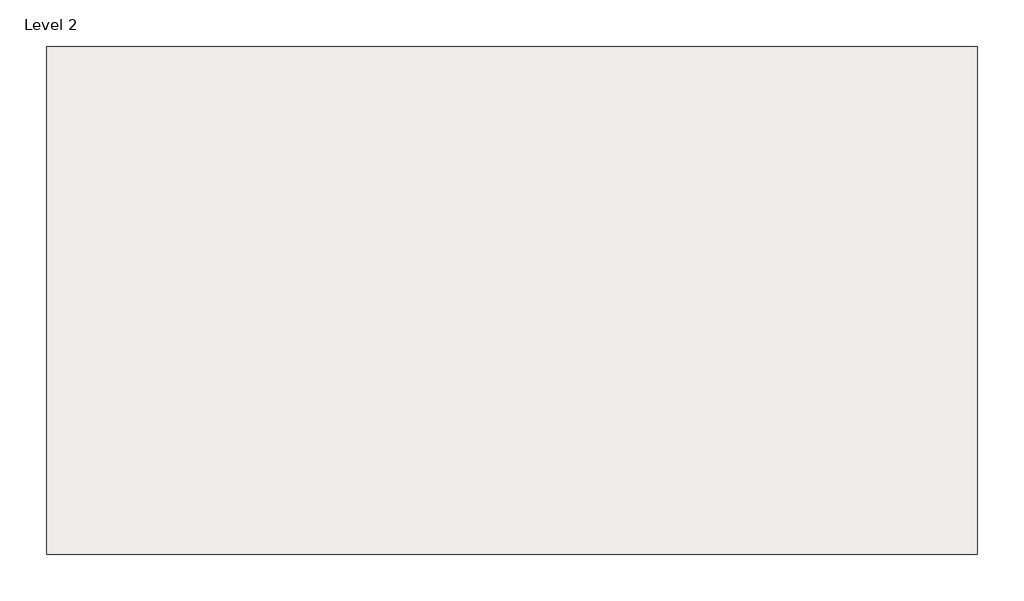
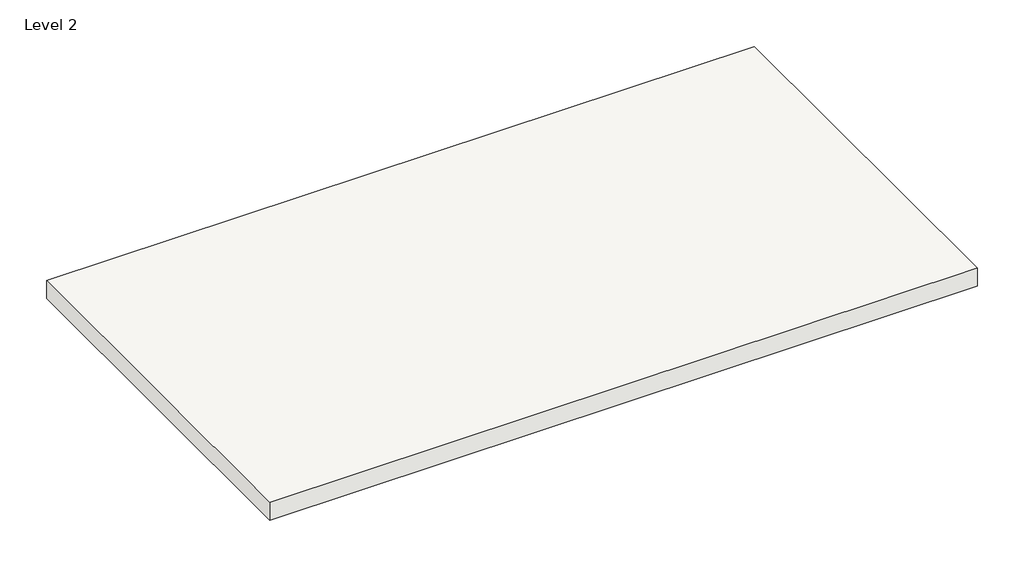
# One storey: 1 roof.
"""IFC4 building model written with IfcOpenShell, lengths in millimetres."""

from ifc_helpers import new_model, si_unit, frame, origin, place, context, project, spatial, polyline, outline, extrude, element, save

model = new_model("IFC4")

# Units and contexts
model_context = context("Model", 3, world=origin())
ifc_project = project(units=[si_unit("LENGTHUNIT", "METRE", prefix="MILLI")], contexts=[model_context])

# Site, building, storey
site = spatial("IfcSite", under=ifc_project)
building = spatial("IfcBuilding", under=site)
storey = spatial("IfcBuildingStorey", under=building, Name="Level 2", Elevation=3048.0)

# Roof
placement = place(None, origin())
element("IfcRoof", 1, ObjectType="Generic - 12\"", at=placement, inside=storey, context=model_context, shape_type="SweptSolid", body=[
    extrude(outline(polyline([(-14311.9118598, 14296.1355643), (-3008.9118598, 14296.1355643), (-3008.9118598, 8123.9355643), (-14311.9118598, 8123.9355643), (-14311.9118598, 14296.1355643)])), frame((0.0, 0.0, 3048.0), z_axis=(0.0, 0.0, 1.0), x_axis=(1.0, 0.0, 0.0)), (0.0, 0.0, 1.0), 304.8),
])

save(model, "model.ifc")

# Revit data of these elements
# Type "Generic - 12\""
#   Assembly Code = "B1020"
#   Layers, outside or top first: 1' - 0" "Brick, Soldier Course" (function 1)
# Element 1 (IfcRoof, "Generic - 12\"")
#   built-in parameter 1001705 = 11 (stored number, unit not read)
#   built-in parameter 1001710 = 33615
#   Phase Created = New Construction
#   Materials on its faces: "Brick, Soldier Course"
# Materials
#   "Brick, Soldier Course": class "Masonry", colour RGB 170 98 104, transparency 0, Description = "Common brick soldier coursed", Cost = 0
